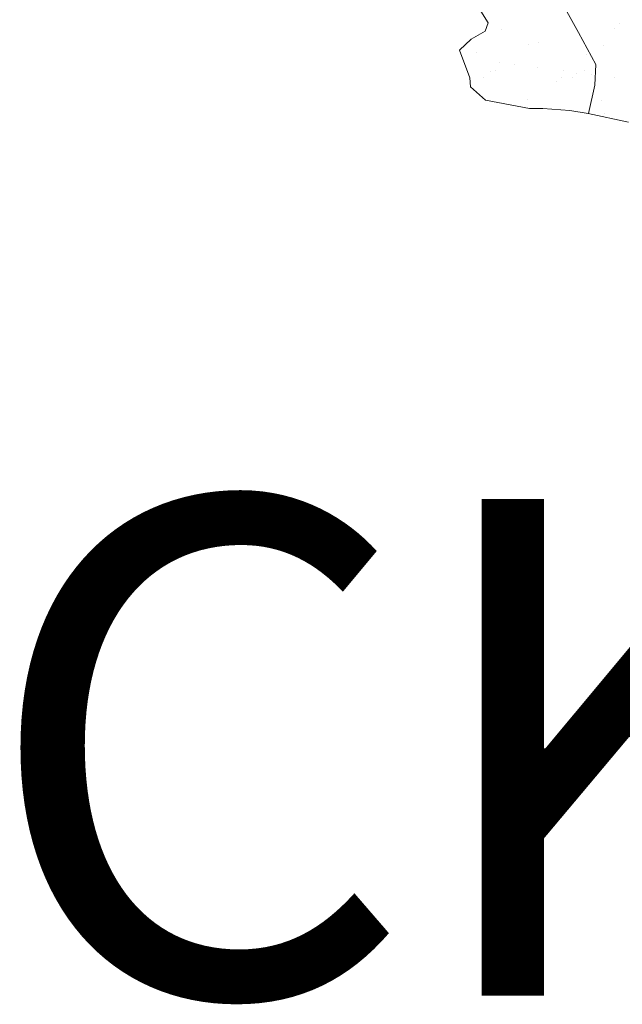
# Model space of a CAD drawing. Units: inches. Extents: x 1986 to 21484, y -1816 to 2016.
# Tile 11 of 85: x 2148.64 to 2157.13, y 1860.02 to 1873.9. Entities that reach past the tile are written whole.
import ezdxf

# ---------------------------------------------------------------- set-up
doc = ezdxf.new("R2010")
doc.units = ezdxf.units.IN
doc.layers.add('A-ANNO-TEXT', color=7, linetype='Continuous', lineweight=18)
doc.layers.add('L-PLNT', color=84, linetype='Continuous', lineweight=13)
doc.styles.get("Standard").update_dxf_attribs({"font": 'arial.ttf'})

# ---------------------------------------------------------------- blocks, each defined once
blk = doc.blocks.new('PLANT-SHRUB')
for p, q in [((2156.514, 1873.716), (2156.28, 1874.139)), ((2155.244, 1873.853), (2155.14, 1874.018)), ((2155.202, 1873.739), (2155.244, 1873.853)), ((2157.101, 1873.84), (2157.101, 1873.84)), ((2155.005, 1873.625), (2155.202, 1873.739)), ((2155.428, 1873.758), (2155.428, 1873.758)), ((2156.762, 1873.265), (2156.514, 1873.716)), ((2157.028, 1873.772), (2157.028, 1873.772)), ((2154.84, 1873.47), (2155.005, 1873.625)), ((2155.005, 1873.625), (2155.005, 1873.625)), ((2155.816, 1873.549), (2155.816, 1873.549)), ((2155.958, 1873.574), (2155.958, 1873.574)), ((2156.862, 1873.535), (2156.862, 1873.535)), ((2154.985, 1873.077), (2154.84, 1873.47)), ((2155.081, 1873.44), (2155.081, 1873.44)), ((2156.63, 1873.408), (2156.63, 1873.408)), ((2155.409, 1873.289), (2155.409, 1873.289)), ((2155.617, 1873.262), (2155.617, 1873.262)), ((2156.746, 1872.977), (2156.762, 1873.265)), ((2155.276, 1873.174), (2155.276, 1873.174)), ((2155.351, 1873.188), (2155.351, 1873.188)), ((2155.942, 1873.219), (2155.942, 1873.219)), ((2156.298, 1873.179), (2156.298, 1873.179)), ((2156.485, 1873.147), (2156.485, 1873.147)), ((2156.596, 1873.186), (2156.596, 1873.186)), ((2156.693, 1873.12), (2156.693, 1873.12)), ((2154.995, 1872.952), (2154.985, 1873.077)), ((2155.183, 1873.081), (2155.183, 1873.081)), ((2156.209, 1873.022), (2156.209, 1873.022)), ((2156.282, 1873.089), (2156.282, 1873.089)), ((2156.427, 1873.078), (2156.427, 1873.078)), ((2156.659, 1872.575), (2156.746, 1872.977)), ((2157.018, 1873.077), (2157.018, 1873.077)), ((2155.203, 1872.763), (2154.995, 1872.952)), ((2155.825, 1872.649), (2155.203, 1872.763)), ((2155.791, 1872.779), (2155.791, 1872.779)), ((2156.837, 1872.765), (2156.837, 1872.765)), ((2156.011, 1872.649), (2155.825, 1872.649)), ((2156.394, 1872.618), (2156.011, 1872.649)), ((2156.653, 1872.576), (2156.394, 1872.618)), ((2157.223, 1872.452), (2156.653, 1872.576)), ((2156.88, 1872.571), (2156.88, 1872.571))]:
    blk.add_line(p, q)

msp = doc.modelspace()

# ---------------------------------------------------------------- block references
at = {"layer": 'L-PLNT'}
msp.add_blockref('PLANT-SHRUB', (0, 0), dxfattribs=at)

# ---------------------------------------------------------------- texts
at = {"layer": 'A-ANNO-TEXT', "insert": (2108.883, 1867.143), "char_height": 7, "attachment_point": 1}
msp.add_mtext_dynamic_manual_height_columns("{\\fTimes New Roman|b0|i0|c0|p18;4' SETBACK}", width=105.61268, gutter_width=12.5, heights=[0], dxfattribs=at)

doc.saveas('drawing.dxf')
